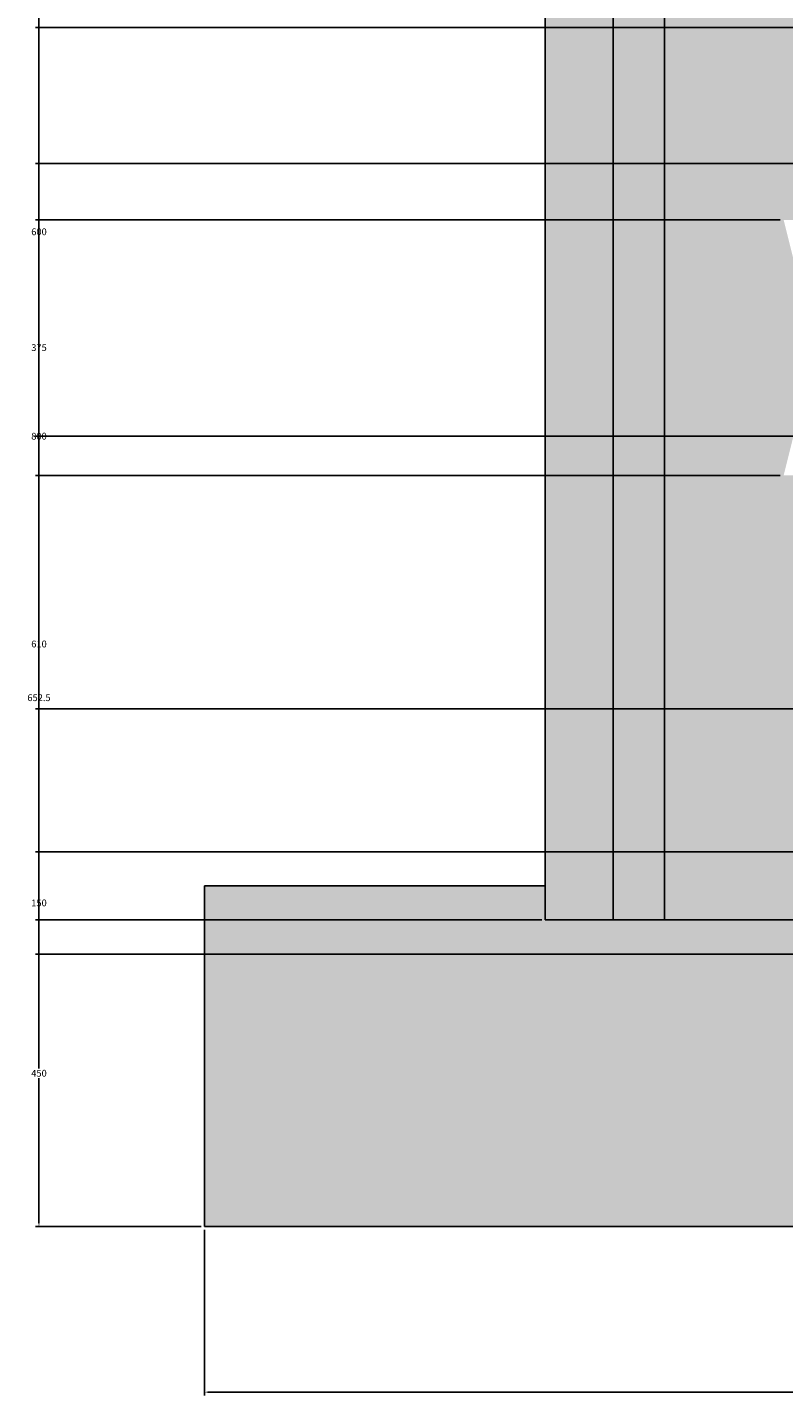
# Model space of a CAD drawing. Units: millimetres. Extents: x 2970 to 7764, y 2196 to 7505.
# Tile 1 of 13: x 2970 to 4081, y 2196 to 4206. Entities that reach past the tile are written whole.
import ezdxf

# ---------------------------------------------------------------- set-up
doc = ezdxf.new("R2010")
doc.units = ezdxf.units.MM
doc.header["$MEASUREMENT"] = 0
for name, color, linetype, lineweight in [('A-ANNO-DIMS', 2, 'Continuous', 18), ('A-ELEV', 7, 'Continuous', 25), ('A-ELEV-PATT', 8, 'Continuous', 13)]:
    doc.layers.add(name, color=color, linetype=linetype, lineweight=lineweight)
doc.styles.get("Standard").update_dxf_attribs({"font": 'arial.ttf'})
doc.dimstyles.get("Standard").update_dxf_attribs({"dimtxt": 10, "dimasz": 5, "dimexe": 5, "dimexo": 5, "dimgap": 2, "dimtad": 0, "dimtih": 1, "dimtoh": 1, "dimdec": 0, "dimzin": 0, "dimdsep": 46, "dimtxsty": 'Standard', "dimcen": 2, "dimadec": 0, "dimazin": 0, "dimtfac": 1, "dimtdec": 0, "dimtofl": 0, "dimtmove": 0, "dimatfit": 3, "dimfxl": 1, "dimtolj": 1, "dimtzin": 0, "dimarcsym": 0})

# ---------------------------------------------------------------- blocks, each defined once
blk = doc.blocks.new('*D10')
at = {"layer": 'A-ANNO-DIMS', "color": 0, "lineweight": -2, "transparency": 16777216}
for p, q in [((3230.5, 2440.8), (3230.5, 2197.8)), ((7505.5, 2440.8), (7505.5, 2197.8)), ((3235.5, 2202.8), (5350.8, 2202.8)), ((7500.5, 2202.8), (5385.2, 2202.8))]:
    blk.add_line(p, q, dxfattribs=at)
at = {"layer": 'A-ANNO-DIMS', "color": 0, "transparency": 16777216}
for points in [[(3235.5, 2203.6), (3235.5, 2202), (3230.5, 2202.8)], [(7500.5, 2203.6), (7500.5, 2202), (7505.5, 2202.8)]]:
    blk.add_solid(points, dxfattribs=at)
at = {"layer": 'Defpoints', "color": 0, "transparency": 16777216}
for p in [(3230.5, 2445.8), (7505.5, 2445.8), (7505.5, 2202.8)]:
    blk.add_point(p, dxfattribs=at)
at = {"layer": 'A-ANNO-DIMS', "color": 0, "transparency": 16777216, "insert": (5368, 2202.8), "char_height": 10, "attachment_point": 5}
blk.add_mtext('\\A1;4275', dxfattribs=at)
blk = doc.blocks.new('*D20')
at = {"layer": 'A-ANNO-DIMS', "color": 0, "lineweight": -2, "transparency": 16777216}
for p, q in [((3725.5, 2895.8), (2982.5, 2895.8)), ((2987.5, 2890.8), (2987.5, 2677.9)), ((2987.5, 2450.8), (2987.5, 2663.7)), ((3225.5, 2445.8), (2982.5, 2445.8))]:
    blk.add_line(p, q, dxfattribs=at)
at = {"layer": 'A-ANNO-DIMS', "color": 0, "transparency": 16777216}
for points in [[(2986.7, 2890.8), (2988.3, 2890.8), (2987.5, 2895.8)], [(2986.7, 2450.8), (2988.3, 2450.8), (2987.5, 2445.8)]]:
    blk.add_solid(points, dxfattribs=at)
at = {"layer": 'Defpoints', "color": 0, "transparency": 16777216}
for p in [(2987.5, 2895.8), (3730.5, 2895.8), (3230.5, 2445.8)]:
    blk.add_point(p, dxfattribs=at)
at = {"layer": 'A-ANNO-DIMS', "color": 0, "transparency": 16777216, "insert": (2987.5, 2670.8), "char_height": 10, "attachment_point": 5}
blk.add_mtext('\\A1;450', dxfattribs=at)
blk = doc.blocks.new('*D21')
at = {"layer": 'A-ANNO-DIMS', "color": 0, "lineweight": -2, "transparency": 16777216}
for p, q in [((4075.5, 3548.3), (2982.5, 3548.3)), ((2987.5, 3543.3), (2987.5, 3229.1)), ((2987.5, 2900.8), (2987.5, 3214.9)), ((3725.5, 2895.8), (2982.5, 2895.8))]:
    blk.add_line(p, q, dxfattribs=at)
at = {"layer": 'A-ANNO-DIMS', "color": 0, "transparency": 16777216}
for points in [[(2986.7, 3543.3), (2988.3, 3543.3), (2987.5, 3548.3)], [(2986.7, 2900.8), (2988.3, 2900.8), (2987.5, 2895.8)]]:
    blk.add_solid(points, dxfattribs=at)
at = {"layer": 'Defpoints', "color": 0, "transparency": 16777216}
for p in [(2987.5, 3548.3), (4080.5, 3548.3), (3730.5, 2895.8)]:
    blk.add_point(p, dxfattribs=at)
at = {"layer": 'A-ANNO-DIMS', "color": 0, "transparency": 16777216, "insert": (2987.5, 3222), "char_height": 10, "attachment_point": 5}
blk.add_mtext('\\A1;652.5', dxfattribs=at)
blk = doc.blocks.new('*D22')
at = {"layer": 'A-ANNO-DIMS', "color": 0, "lineweight": -2, "transparency": 16777216}
for p, q in [((4075.5, 3923.3), (2982.5, 3923.3)), ((2987.5, 3918.3), (2987.5, 3742.9)), ((2987.5, 3553.3), (2987.5, 3728.7)), ((4075.5, 3548.3), (2982.5, 3548.3))]:
    blk.add_line(p, q, dxfattribs=at)
at = {"layer": 'A-ANNO-DIMS', "color": 0, "transparency": 16777216}
for points in [[(2986.7, 3918.3), (2988.3, 3918.3), (2987.5, 3923.3)], [(2986.7, 3553.3), (2988.3, 3553.3), (2987.5, 3548.3)]]:
    blk.add_solid(points, dxfattribs=at)
at = {"layer": 'Defpoints', "color": 0, "transparency": 16777216}
for p in [(2987.5, 3923.3), (4080.5, 3923.3), (4080.5, 3548.3)]:
    blk.add_point(p, dxfattribs=at)
at = {"layer": 'A-ANNO-DIMS', "color": 0, "transparency": 16777216, "insert": (2987.5, 3735.8), "char_height": 10, "attachment_point": 5}
blk.add_mtext('\\A1;375', dxfattribs=at)
blk = doc.blocks.new('*D23')
at = {"layer": 'A-ANNO-DIMS', "color": 0, "lineweight": -2, "transparency": 16777216}
for p, q in [((4075.5, 5228.3), (2982.5, 5228.3)), ((2987.5, 5223.3), (2987.5, 4582.9)), ((2987.5, 3928.3), (2987.5, 4568.7)), ((4075.5, 3923.3), (2982.5, 3923.3))]:
    blk.add_line(p, q, dxfattribs=at)
at = {"layer": 'A-ANNO-DIMS', "color": 0, "transparency": 16777216}
for points in [[(2986.7, 5223.3), (2988.3, 5223.3), (2987.5, 5228.3)], [(2986.7, 3928.3), (2988.3, 3928.3), (2987.5, 3923.3)]]:
    blk.add_solid(points, dxfattribs=at)
at = {"layer": 'Defpoints', "color": 0, "transparency": 16777216}
for p in [(2987.5, 5228.3), (4080.5, 5228.3), (4080.5, 3923.3)]:
    blk.add_point(p, dxfattribs=at)
at = {"layer": 'A-ANNO-DIMS', "color": 0, "transparency": 16777216, "insert": (2987.5, 4575.8), "char_height": 10, "attachment_point": 5}
blk.add_mtext('\\A1;1305', dxfattribs=at)
blk = doc.blocks.new('*D44')
at = {"layer": 'A-ANNO-DIMS', "color": 0, "lineweight": -2, "transparency": 16777216}
for p, q in [((4350.5, 2995.8), (2982.5, 2995.8)), ((2987.5, 2990.8), (2987.5, 2927.9)), ((2987.5, 2850.8), (2987.5, 2913.7)), ((4350.5, 2845.8), (2982.5, 2845.8))]:
    blk.add_line(p, q, dxfattribs=at)
at = {"layer": 'A-ANNO-DIMS', "color": 0, "transparency": 16777216}
for points in [[(2986.7, 2990.8), (2988.3, 2990.8), (2987.5, 2995.8)], [(2986.7, 2850.8), (2988.3, 2850.8), (2987.5, 2845.8)]]:
    blk.add_solid(points, dxfattribs=at)
at = {"layer": 'Defpoints', "color": 0, "transparency": 16777216}
for p in [(2987.5, 2995.8), (4355.5, 2995.8), (4355.5, 2845.8)]:
    blk.add_point(p, dxfattribs=at)
at = {"layer": 'A-ANNO-DIMS', "color": 0, "transparency": 16777216, "insert": (2987.5, 2920.8), "char_height": 10, "attachment_point": 5}
blk.add_mtext('\\A1;150', dxfattribs=at)
blk = doc.blocks.new('*D45')
at = {"layer": 'A-ANNO-DIMS', "color": 0, "lineweight": -2, "transparency": 16777216}
for p, q in [((4880.5, 3605.8), (2982.5, 3605.8)), ((2987.5, 3600.8), (2987.5, 3307.9)), ((2987.5, 3000.8), (2987.5, 3293.7)), ((4350.5, 2995.8), (2982.5, 2995.8))]:
    blk.add_line(p, q, dxfattribs=at)
at = {"layer": 'A-ANNO-DIMS', "color": 0, "transparency": 16777216}
for points in [[(2986.7, 3600.8), (2988.3, 3600.8), (2987.5, 3605.8)], [(2986.7, 3000.8), (2988.3, 3000.8), (2987.5, 2995.8)]]:
    blk.add_solid(points, dxfattribs=at)
at = {"layer": 'Defpoints', "color": 0, "transparency": 16777216}
for p in [(2987.5, 3605.8), (4885.5, 3605.8), (4355.5, 2995.8)]:
    blk.add_point(p, dxfattribs=at)
at = {"layer": 'A-ANNO-DIMS', "color": 0, "transparency": 16777216, "insert": (2987.5, 3300.8), "char_height": 10, "attachment_point": 5}
blk.add_mtext('\\A1;610', dxfattribs=at)
blk = doc.blocks.new('*D46')
at = {"layer": 'A-ANNO-DIMS', "color": 0, "lineweight": -2, "transparency": 16777216}
for p, q in [((4350.5, 4205.8), (2982.5, 4205.8)), ((2987.5, 4200.8), (2987.5, 3912.9)), ((2987.5, 3610.8), (2987.5, 3898.7)), ((4880.5, 3605.8), (2982.5, 3605.8))]:
    blk.add_line(p, q, dxfattribs=at)
at = {"layer": 'A-ANNO-DIMS', "color": 0, "transparency": 16777216}
for points in [[(2986.7, 4200.8), (2988.3, 4200.8), (2987.5, 4205.8)], [(2986.7, 3610.8), (2988.3, 3610.8), (2987.5, 3605.8)]]:
    blk.add_solid(points, dxfattribs=at)
at = {"layer": 'Defpoints', "color": 0, "transparency": 16777216}
for p in [(2987.5, 4205.8), (4355.5, 4205.8), (4885.5, 3605.8)]:
    blk.add_point(p, dxfattribs=at)
at = {"layer": 'A-ANNO-DIMS', "color": 0, "transparency": 16777216, "insert": (2987.5, 3905.8), "char_height": 10, "attachment_point": 5}
blk.add_mtext('\\A1;600', dxfattribs=at)
blk = doc.blocks.new('*D49')
at = {"layer": 'A-ANNO-DIMS', "color": 0, "lineweight": -2, "transparency": 16777216}
for p, q in [((5950.3, 4005.8), (2982.5, 4005.8)), ((2987.5, 4000.8), (2987.5, 3612.9)), ((2987.5, 3210.8), (2987.5, 3598.7)), ((5950.3, 3205.8), (2982.5, 3205.8))]:
    blk.add_line(p, q, dxfattribs=at)
at = {"layer": 'A-ANNO-DIMS', "color": 0, "transparency": 16777216}
for points in [[(2986.7, 4000.8), (2988.3, 4000.8), (2987.5, 4005.8)], [(2986.7, 3210.8), (2988.3, 3210.8), (2987.5, 3205.8)]]:
    blk.add_solid(points, dxfattribs=at)
at = {"layer": 'Defpoints', "color": 0, "transparency": 16777216}
for p in [(2987.5, 4005.8), (5955.3, 4005.8), (5955.3, 3205.8)]:
    blk.add_point(p, dxfattribs=at)
at = {"layer": 'A-ANNO-DIMS', "color": 0, "transparency": 16777216, "insert": (2987.5, 3605.8), "char_height": 10, "attachment_point": 5}
blk.add_mtext('\\A1;800', dxfattribs=at)

msp = doc.modelspace()

# ---------------------------------------------------------------- hatches: boundary and pattern name
at = {"layer": 'A-ELEV-PATT'}
h = msp.add_hatch(color=256, dxfattribs=at)
h.dxf.hatch_style = 1
h.paths.add_polyline_path([(6405.5, 7255.789), (4305.5, 7255.789), (4305.5, 6505.789), (3730.5, 6505.789), (3730.5, 4205.789), (3730.5, 2945.789), (3730.5, 2895.789), (3830.5, 2895.789), (3830.5, 4205.789), (3830.5, 6405.789), (4405.5, 6405.789), (4405.5, 4205.789), (6905.5, 4205.789), (6905.5, 2945.789), (6905.5, 2845.789), (7155.5, 2845.789), (7155.5, 2945.789), (7155.5, 4205.789), (7155.5, 4455.789), (4555.5, 4455.789), (4555.5, 6505.789), (4555.5, 7005.789), (6155.5, 7005.789), (6155.5, 6755.789), (6405.5, 6755.789)])
h.paths.add_polyline_path([(7405.5, 6755.789), (6155.5, 6755.789), (5755.5, 6755.789), (5755.5, 5005.789), (7405.5, 5005.789)])
h.paths.add_polyline_path([(7155.5, 6505.789), (7155.5, 5255.789), (6005.5, 5255.789), (6005.5, 6505.789)], flags=16)
h.paths.add_polyline_path([(6105.5, 5520.789), (6105.5, 6055.789), (6455.5, 6055.789), (6455.5, 5520.789), (6655.5, 5520.789), (6655.5, 5605.789), (6655.5, 5955.789), (6955.5, 5955.789), (6955.5, 5605.789), (6955.5, 5520.789)], flags=0)
h.paths.add_polyline_path([(6425.5, 5755.789), (6425.5, 5655.789), (6425.5, 5555.789), (6405.5, 5555.789), (6405.5, 5755.789)], flags=0)
h.paths.add_polyline_path([(6955.5, 5505.789), (6955.5, 5405.789), (6655.5, 5405.789), (6655.5, 5505.789)], flags=0)
h = msp.add_hatch(color=256, dxfattribs=at)
h.set_gradient(color1=(76, 38, 38), color2=(99, 100, 102), name='INVSPHERICAL')
h.paths.add_polyline_path([(3830.5, 6405.789), (3830.5, 4205.789), (3830.5, 2895.789), (3905.5, 2895.789), (3905.5, 4205.789), (3905.5, 6255.789), (4405.5, 6255.789), (4405.5, 6405.789)])
h = msp.add_hatch(color=256, dxfattribs=at)
h.set_gradient(color1=(53, 53, 54), color2=(99, 100, 102), name='SPHERICAL')
h.paths.add_polyline_path([(4405.5, 6255.789), (3905.5, 6255.789), (3905.5, 4205.789), (3905.5, 2895.789), (4355.5, 2895.789), (4355.5, 2995.799, -0.50803883), (4340.162, 3038.75, -0.52056705), (4337.177, 3086.472, -0.19797947), (4355.5, 3108.072), (4355.5, 4205.789), (4405.5, 4205.789)])
h.paths.add_polyline_path([(4080.5, 5228.289), (4105.5, 5328.289), (4105.5, 5503.289), (4080.5, 5603.289), (4230.5, 5603.289), (4205.5, 5503.289), (4205.5, 5328.289), (4230.5, 5228.289)], flags=16)
h.paths.add_polyline_path([(4120.5, 5343.289), (4120.5, 5488.289), (4190.5, 5488.289), (4190.5, 5343.289)], flags=0)
h.paths.add_polyline_path([(4230.5, 3923.289), (4205.5, 3823.289), (4205.5, 3648.289), (4230.5, 3548.289), (4080.5, 3548.289), (4105.5, 3648.289), (4105.5, 3823.289), (4080.5, 3923.289)], flags=16)
h.paths.add_polyline_path([(4190.5, 3808.289), (4190.5, 3663.289), (4120.5, 3663.289), (4120.5, 3808.289)], flags=0)
h = msp.add_hatch(color=256, dxfattribs=at)
h.dxf.hatch_style = 1
h.paths.add_polyline_path([(7505.5, 2945.789), (7155.5, 2945.789), (7155.5, 2845.789), (6905.5, 2845.789), (4355.5, 2845.789), (4355.5, 2895.789), (3730.5, 2895.789), (3730.5, 2945.789), (3230.5, 2945.789), (3230.5, 2445.789), (7505.5, 2445.789)])

# ---------------------------------------------------------------- linework, layer by layer
at = {"layer": 'A-ELEV'}
for p, q in [((3730.5, 4205.789), (3730.5, 6505.789)), ((3830.5, 4205.789), (3830.5, 6405.789)), ((3905.5, 4205.789), (3905.5, 6255.789)), ((3730.5, 2945.789), (3730.5, 4205.789)), ((3830.5, 2895.789), (3830.5, 4205.789)), ((3905.5, 2895.789), (3905.5, 4205.789)), ((3230.5, 2445.789), (3230.5, 2945.789)), ((3230.5, 2945.789), (3730.5, 2945.789)), ((3730.5, 2895.789), (3730.5, 2945.789)), ((4355.5, 2895.789), (3730.5, 2895.789)), ((7505.5, 2445.789), (3230.5, 2445.789))]:
    msp.add_line(p, q, dxfattribs=at)

# ---------------------------------------------------------------- dimensions: what is measured, and where the dimension line sits
at = {"layer": 'A-ANNO-DIMS'}
for base, p1, p2, override, picture, middle in [((2987.5, 5228.289), (4080.5, 3923.289), (4080.5, 5228.289), {"dimdec": 0, "dimlfac": 1, "dimrnd": 0, "dimzin": 0, "dimdsep": 46, "dimlunit": 2}, '*D23', (2987.5, 4575.789)), ((2987.5, 4205.789), (4885.5, 3605.789), (4355.5, 4205.789), {"dimdec": 0, "dimlfac": 1, "dimrnd": 0, "dimzin": 0, "dimdsep": 46, "dimlunit": 2}, '*D46', (2987.5, 3905.789)), ((2987.5, 4005.789), (5955.271, 3205.789), (5955.271, 4005.789), {"dimdec": 0, "dimlfac": 1, "dimrnd": 0, "dimzin": 0, "dimdsep": 46, "dimlunit": 2}, '*D49', (2987.5, 3605.789)), ((2987.5, 3923.289), (4080.5, 3548.289), (4080.5, 3923.289), {"dimdec": 0, "dimlfac": 1, "dimrnd": 0, "dimzin": 0, "dimdsep": 46, "dimlunit": 2}, '*D22', (2987.5, 3735.789)), ((2987.5, 3605.789), (4355.5, 2995.789), (4885.5, 3605.789), {"dimdec": 0, "dimlfac": 1, "dimrnd": 0, "dimzin": 0, "dimdsep": 46, "dimlunit": 2}, '*D45', (2987.5, 3300.789)), ((2987.5, 3548.289), (3730.5, 2895.789), (4080.5, 3548.289), {"dimdec": 1, "dimlfac": 1, "dimrnd": 0, "dimzin": 0, "dimdsep": 46, "dimlunit": 2}, '*D21', (2987.5, 3222.039)), ((2987.5, 2995.789), (4355.5, 2845.789), (4355.5, 2995.789), {"dimdec": 0, "dimlfac": 1, "dimrnd": 0, "dimzin": 0, "dimdsep": 46, "dimlunit": 2}, '*D44', (2987.5, 2920.789)), ((2987.5, 2895.789), (3230.5, 2445.789), (3730.5, 2895.789), {"dimdec": 0, "dimlfac": 1, "dimrnd": 0, "dimzin": 0, "dimdsep": 46, "dimlunit": 2}, '*D20', (2987.5, 2670.789))]:
    dim = msp.add_linear_dim(base=base, p1=p1, p2=p2, angle=90, dimstyle='Standard', override=override, dxfattribs=at)
    dim.commit()
    dim.dimension.update_dxf_attribs({"geometry": picture, "text_midpoint": middle})
dim = msp.add_linear_dim(base=(7505.5, 2202.789), p1=(3230.5, 2445.789), p2=(7505.5, 2445.789), dimstyle='Standard', override={"dimdec": 0, "dimlfac": 1, "dimrnd": 0, "dimzin": 0, "dimdsep": 46, "dimlunit": 2}, dxfattribs=at)
dim.commit()
dim.dimension.update_dxf_attribs({"geometry": '*D10', "text_midpoint": (5368, 2202.789)})

doc.saveas('drawing.dxf')
